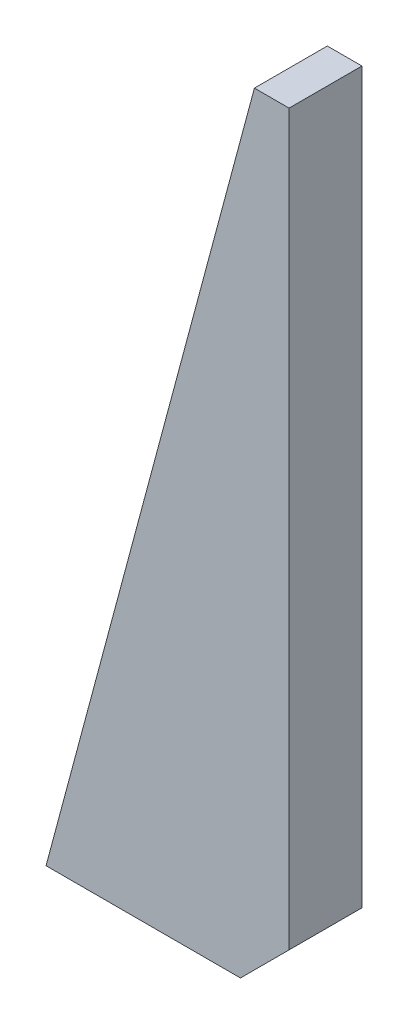
ISO-10303-21;
HEADER;
FILE_DESCRIPTION(('STEP AP214'),'2;1');
FILE_NAME('part.step','',(''),(''),'','','');
FILE_SCHEMA(('AUTOMOTIVE_DESIGN { 1 0 10303 214 1 1 1 1 }'));
ENDSEC;
DATA;
#1=APPLICATION_CONTEXT('core data for automotive mechanical design processes');
#2=APPLICATION_PROTOCOL_DEFINITION('international standard','automotive_design',2000,#1);
#3=PRODUCT_CONTEXT('',#1,'mechanical');
#4=PRODUCT('Part','Part','',(#3));
#5=PRODUCT_RELATED_PRODUCT_CATEGORY('part','',(#4));
#6=PRODUCT_DEFINITION_FORMATION('','',#4);
#7=PRODUCT_DEFINITION_CONTEXT('part definition',#1,'design');
#8=PRODUCT_DEFINITION('design','',#6,#7);
#9=PRODUCT_DEFINITION_SHAPE('','',#8);
#10=(LENGTH_UNIT() NAMED_UNIT(*) SI_UNIT(.MILLI.,.METRE.));
#11=(NAMED_UNIT(*) PLANE_ANGLE_UNIT() SI_UNIT($,.RADIAN.));
#12=(NAMED_UNIT(*) SI_UNIT($,.STERADIAN.) SOLID_ANGLE_UNIT());
#13=UNCERTAINTY_MEASURE_WITH_UNIT(LENGTH_MEASURE(1.E-05),#10,'distance_accuracy_value','');
#14=(GEOMETRIC_REPRESENTATION_CONTEXT(3) GLOBAL_UNCERTAINTY_ASSIGNED_CONTEXT((#13)) GLOBAL_UNIT_ASSIGNED_CONTEXT((#10,
#11,#12)) REPRESENTATION_CONTEXT('',''));
#15=CARTESIAN_POINT('',(0.,0.,0.));
#16=DIRECTION('',(0.,0.,1.));
#17=DIRECTION('',(1.,0.,0.));
#18=AXIS2_PLACEMENT_3D('',#15,#16,#17);
#19=CARTESIAN_POINT('',(0.,160.,15.));
#20=DIRECTION('',(-1.,0.,0.));
#21=DIRECTION('',(0.,0.,1.));
#22=AXIS2_PLACEMENT_3D('',#19,#20,#21);
#23=PLANE('',#22);
#24=DIRECTION('',(0.,1.,0.));
#25=VECTOR('',#24,1.);
#26=CARTESIAN_POINT('',(0.,160.,15.));
#27=LINE('',#26,#25);
#28=CARTESIAN_POINT('',(0.,9.99999999999998,15.));
#29=VERTEX_POINT('',#28);
#30=CARTESIAN_POINT('',(0.,160.,15.));
#31=VERTEX_POINT('',#30);
#32=EDGE_CURVE('E86',#29,#31,#27,.T.);
#33=ORIENTED_EDGE('',*,*,#32,.F.);
#34=DIRECTION('',(0.,0.,-1.));
#35=VECTOR('',#34,1.);
#36=CARTESIAN_POINT('',(0.,9.99999999999998,15.));
#37=LINE('',#36,#35);
#38=CARTESIAN_POINT('',(0.,9.99999999999998,0.));
#39=VERTEX_POINT('',#38);
#40=EDGE_CURVE('E112',#29,#39,#37,.T.);
#41=ORIENTED_EDGE('',*,*,#40,.T.);
#42=DIRECTION('',(0.,1.,0.));
#43=VECTOR('',#42,1.);
#44=CARTESIAN_POINT('',(0.,160.,0.));
#45=LINE('',#44,#43);
#46=CARTESIAN_POINT('',(0.,160.,0.));
#47=VERTEX_POINT('',#46);
#48=EDGE_CURVE('E108',#39,#47,#45,.T.);
#49=ORIENTED_EDGE('',*,*,#48,.T.);
#50=DIRECTION('',(0.,0.,-1.));
#51=VECTOR('',#50,1.);
#52=CARTESIAN_POINT('',(0.,160.,15.));
#53=LINE('',#52,#51);
#54=EDGE_CURVE('E103',#31,#47,#53,.T.);
#55=ORIENTED_EDGE('',*,*,#54,.F.);
#56=EDGE_LOOP('',(#33,#41,#49,#55));
#57=FACE_BOUND('',#56,.T.);
#58=ADVANCED_FACE('F41',(#57),#23,.F.);
#59=CARTESIAN_POINT('',(-7.1281292110197,160.,15.));
#60=DIRECTION('',(0.,-1.,0.));
#61=DIRECTION('',(0.,0.,-1.));
#62=AXIS2_PLACEMENT_3D('',#59,#60,#61);
#63=PLANE('',#62);
#64=DIRECTION('',(-1.,0.,0.));
#65=VECTOR('',#64,1.);
#66=CARTESIAN_POINT('',(-7.1281292110197,160.,0.));
#67=LINE('',#66,#65);
#68=CARTESIAN_POINT('',(-7.1281292110197,160.,0.));
#69=VERTEX_POINT('',#68);
#70=EDGE_CURVE('E123',#47,#69,#67,.T.);
#71=ORIENTED_EDGE('',*,*,#70,.T.);
#72=DIRECTION('',(0.,0.,-1.));
#73=VECTOR('',#72,1.);
#74=CARTESIAN_POINT('',(-7.1281292110197,160.,15.));
#75=LINE('',#74,#73);
#76=CARTESIAN_POINT('',(-7.1281292110197,160.,15.));
#77=VERTEX_POINT('',#76);
#78=EDGE_CURVE('E104',#77,#69,#75,.T.);
#79=ORIENTED_EDGE('',*,*,#78,.F.);
#80=DIRECTION('',(-1.,0.,0.));
#81=VECTOR('',#80,1.);
#82=CARTESIAN_POINT('',(-7.1281292110197,160.,15.));
#83=LINE('',#82,#81);
#84=EDGE_CURVE('E93',#31,#77,#83,.T.);
#85=ORIENTED_EDGE('',*,*,#84,.F.);
#86=ORIENTED_EDGE('',*,*,#54,.T.);
#87=EDGE_LOOP('',(#71,#79,#85,#86));
#88=FACE_BOUND('',#87,.T.);
#89=ADVANCED_FACE('F105',(#88),#63,.F.);
#90=CARTESIAN_POINT('',(-50.,0.,15.));
#91=DIRECTION('',(0.965925826289067,-0.258819045102525,0.));
#92=DIRECTION('',(0.258819045102525,0.965925826289067,0.));
#93=AXIS2_PLACEMENT_3D('',#90,#91,#92);
#94=PLANE('',#93);
#95=DIRECTION('',(-0.258819045102525,-0.965925826289067,0.));
#96=VECTOR('',#95,1.);
#97=CARTESIAN_POINT('',(-50.,0.,0.));
#98=LINE('',#97,#96);
#99=CARTESIAN_POINT('',(-50.,0.,0.));
#100=VERTEX_POINT('',#99);
#101=EDGE_CURVE('E122',#69,#100,#98,.T.);
#102=ORIENTED_EDGE('',*,*,#101,.T.);
#103=DIRECTION('',(0.,0.,-1.));
#104=VECTOR('',#103,1.);
#105=CARTESIAN_POINT('',(-50.,0.,15.));
#106=LINE('',#105,#104);
#107=CARTESIAN_POINT('',(-50.,0.,15.));
#108=VERTEX_POINT('',#107);
#109=EDGE_CURVE('E111',#108,#100,#106,.T.);
#110=ORIENTED_EDGE('',*,*,#109,.F.);
#111=DIRECTION('',(-0.258819045102525,-0.965925826289067,0.));
#112=VECTOR('',#111,1.);
#113=CARTESIAN_POINT('',(-50.,0.,15.));
#114=LINE('',#113,#112);
#115=EDGE_CURVE('E110',#77,#108,#114,.T.);
#116=ORIENTED_EDGE('',*,*,#115,.F.);
#117=ORIENTED_EDGE('',*,*,#78,.T.);
#118=EDGE_LOOP('',(#102,#110,#116,#117));
#119=FACE_BOUND('',#118,.T.);
#120=ADVANCED_FACE('F128',(#119),#94,.F.);
#121=CARTESIAN_POINT('',(0.,0.,15.));
#122=DIRECTION('',(0.,1.,0.));
#123=DIRECTION('',(-1.,0.,0.));
#124=AXIS2_PLACEMENT_3D('',#121,#122,#123);
#125=PLANE('',#124);
#126=DIRECTION('',(1.,0.,0.));
#127=VECTOR('',#126,1.);
#128=CARTESIAN_POINT('',(0.,0.,0.));
#129=LINE('',#128,#127);
#130=CARTESIAN_POINT('',(-10.,0.,0.));
#131=VERTEX_POINT('',#130);
#132=EDGE_CURVE('E98',#100,#131,#129,.T.);
#133=ORIENTED_EDGE('',*,*,#132,.T.);
#134=DIRECTION('',(0.,0.,1.));
#135=VECTOR('',#134,1.);
#136=CARTESIAN_POINT('',(-10.,0.,15.));
#137=LINE('',#136,#135);
#138=CARTESIAN_POINT('',(-10.,0.,15.));
#139=VERTEX_POINT('',#138);
#140=EDGE_CURVE('E49',#131,#139,#137,.T.);
#141=ORIENTED_EDGE('',*,*,#140,.T.);
#142=DIRECTION('',(1.,0.,0.));
#143=VECTOR('',#142,1.);
#144=CARTESIAN_POINT('',(0.,0.,15.));
#145=LINE('',#144,#143);
#146=EDGE_CURVE('E116',#108,#139,#145,.T.);
#147=ORIENTED_EDGE('',*,*,#146,.F.);
#148=ORIENTED_EDGE('',*,*,#109,.T.);
#149=EDGE_LOOP('',(#133,#141,#147,#148));
#150=FACE_BOUND('',#149,.T.);
#151=ADVANCED_FACE('F134',(#150),#125,.F.);
#152=CARTESIAN_POINT('',(0.,0.,15.));
#153=DIRECTION('',(0.,0.,-1.));
#154=DIRECTION('',(-1.,0.,0.));
#155=AXIS2_PLACEMENT_3D('',#152,#153,#154);
#156=PLANE('',#155);
#157=ORIENTED_EDGE('',*,*,#146,.T.);
#158=DIRECTION('',(-0.707106781186548,-0.707106781186547,0.));
#159=VECTOR('',#158,1.);
#160=CARTESIAN_POINT('',(0.,9.99999999999998,15.));
#161=LINE('',#160,#159);
#162=EDGE_CURVE('E11',#139,#29,#161,.F.);
#163=ORIENTED_EDGE('',*,*,#162,.T.);
#164=ORIENTED_EDGE('',*,*,#32,.T.);
#165=ORIENTED_EDGE('',*,*,#84,.T.);
#166=ORIENTED_EDGE('',*,*,#115,.T.);
#167=EDGE_LOOP('',(#157,#163,#164,#165,#166));
#168=FACE_BOUND('',#167,.T.);
#169=ADVANCED_FACE('F89',(#168),#156,.F.);
#170=CARTESIAN_POINT('',(0.,0.,0.));
#171=DIRECTION('',(0.,0.,-1.));
#172=DIRECTION('',(-1.,0.,0.));
#173=AXIS2_PLACEMENT_3D('',#170,#171,#172);
#174=PLANE('',#173);
#175=ORIENTED_EDGE('',*,*,#48,.F.);
#176=DIRECTION('',(0.707106781186548,0.707106781186547,0.));
#177=VECTOR('',#176,1.);
#178=CARTESIAN_POINT('',(-4.99999999999999,5.,0.));
#179=LINE('',#178,#177);
#180=EDGE_CURVE('E65',#39,#131,#179,.F.);
#181=ORIENTED_EDGE('',*,*,#180,.T.);
#182=ORIENTED_EDGE('',*,*,#132,.F.);
#183=ORIENTED_EDGE('',*,*,#101,.F.);
#184=ORIENTED_EDGE('',*,*,#70,.F.);
#185=EDGE_LOOP('',(#175,#181,#182,#183,#184));
#186=FACE_BOUND('',#185,.T.);
#187=ADVANCED_FACE('F138',(#186),#174,.T.);
#188=CARTESIAN_POINT('',(0.,9.99999999999998,15.));
#189=DIRECTION('',(-0.707106781186547,0.707106781186548,0.));
#190=DIRECTION('',(0.,0.,-1.));
#191=AXIS2_PLACEMENT_3D('',#188,#189,#190);
#192=PLANE('',#191);
#193=ORIENTED_EDGE('',*,*,#162,.F.);
#194=ORIENTED_EDGE('',*,*,#140,.F.);
#195=ORIENTED_EDGE('',*,*,#180,.F.);
#196=ORIENTED_EDGE('',*,*,#40,.F.);
#197=EDGE_LOOP('',(#193,#194,#195,#196));
#198=FACE_BOUND('',#197,.T.);
#199=ADVANCED_FACE('F42',(#198),#192,.F.);
#200=CLOSED_SHELL('',(#58,#89,#120,#151,#169,#187,#199));
#201=MANIFOLD_SOLID_BREP('B2',#200);
#202=ADVANCED_BREP_SHAPE_REPRESENTATION('',(#18,#201),#14);
#203=SHAPE_DEFINITION_REPRESENTATION(#9,#202);
ENDSEC;
END-ISO-10303-21;
